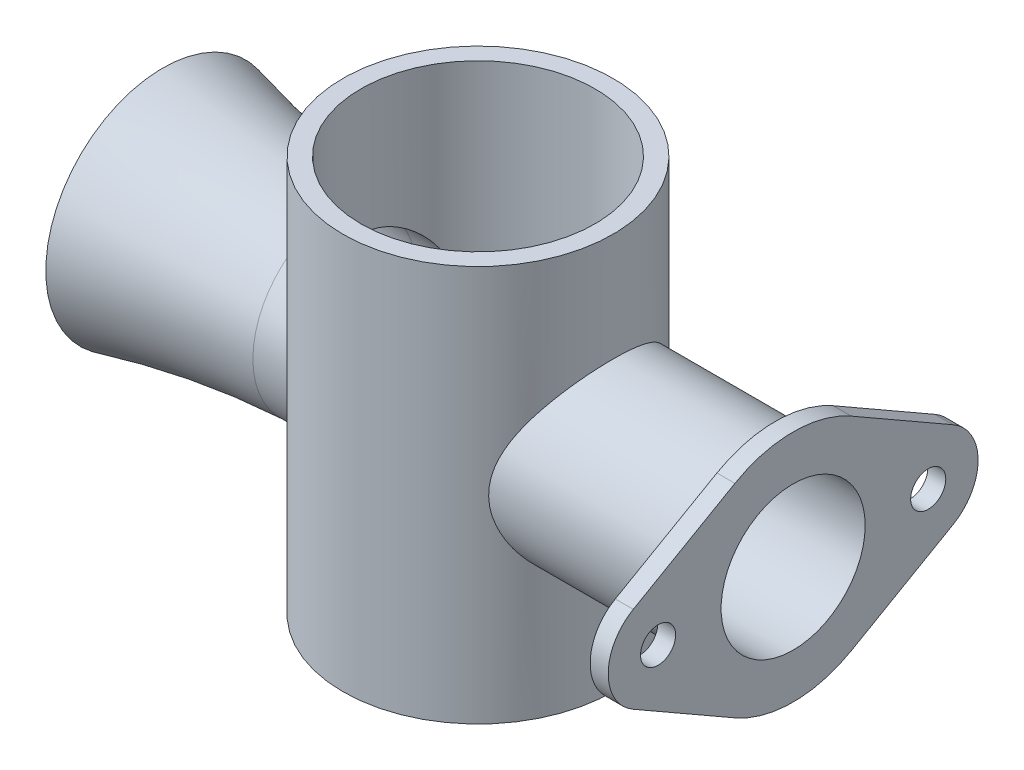
SolidWorks part; units mm, degrees
material "Plain Carbon Steel"
ref_plane "Front Plane" through (0, 0, 0) normal (0, 0, 1) x (1, 0, 0)
ref_plane "Top Plane" through (0, 0, 0) normal (0, 1, 0) x (1, 0, 0)
ref_plane "Right Plane" through (0, 0, 0) normal (1, 0, 0) x (0, 0, -1)
sketch "Main Barrel Sketch" plane through (0, 0, 0) normal (0, 1, 0) x (1, 0, 0)
  circle A0 centre (0, 0) radius 7.5
  circle A1 centre (0, 0) radius 6.5
  dimension "D1" = 15
  dimension "D2" = 13
extrude "Main Barrel" add sketch "Main Barrel Sketch" along normal mid plane 22 contours A0
sketch "Main Bore Sketch Ø13" plane through (0, 11, 0) normal (0, 1, 0) x (1, 0, 0)
  circle A0 centre (0, 0) radius 6.5
  dimension "D1" = 13
extrude "Main Bore Ø13" cut sketch "Main Bore Sketch Ø13" against normal blind 20
ref_plane "Outlet Tube Plane" through (7.5, 0, 0) normal (-1, 0, 0) x (0, 0, 1)
sketch "Outlet Tube Sketch Ø10" plane through (7.5, 0, 0) normal (-1, 0, 0) x (0, 0, 1)
  circle A0 centre (0, 0) radius 5
  dimension "D1" = 10
extrude "Outlet Tube Ø10" add sketch "Outlet Tube Sketch Ø10" against normal blind 9 separate body
sketch "Mounting Flange Sketch" plane through (16.5, 0, 0) normal (1, 0, 0) x (0, 0, -1)
  line L0 (-12.9164, 0) -> (13.3464, 0) construction
  line L1 (-7.5, 11) -> (-7.5, -11) construction
  line L2 (7.5, 11) -> (7.5, -11) construction
  line L3 (0, -9.8134) -> (0, 13.4745) construction
  line L4 (3.2327, 5.6391) -> (8.8776, 2.4031)
  line L5 (3.2327, -5.6391) -> (8.8776, -2.4031)
  line L6 (-3.2327, -5.6391) -> (-8.8776, -2.4031)
  line L7 (-3.2327, 5.6391) -> (-8.8776, 2.4031)
  circle A0 centre (0, 0) radius 4
  arc A1 (3.2327, 5.6391) -> (-3.2327, 5.6391) centre (0, 0) ccw
  circle A2 centre (7.5, 0) radius 0.975
  arc A3 (8.8776, -2.4031) -> (8.8776, 2.4031) centre (7.5, 0) ccw
  arc A4 (-8.8776, -2.4031) -> (-8.8776, 2.4031) centre (-7.5, 0) cw
  arc A5 (-3.2327, -5.6391) -> (3.2327, -5.6391) centre (0, 0) ccw
  circle A6 centre (-7.5, 0) radius 0.975
  dimension "D1" = 8
  dimension "D2" = 13
  dimension "D3" = 1.95
  dimension "D4" = 5.54
extrude "Mounting Flange" add sketch "Mounting Flange Sketch" along normal blind 1
sketch "Outlet Tube Joint Sketch" plane through (7.5, 0, 0) normal (-1, 0, 0) x (0, 0, 1)
  circle A0 centre (0, 0) radius 5 construction
  circle A1 centre (0, 0) radius 5
extrude "Outlet Tube Joint" add sketch "Outlet Tube Joint Sketch" along normal up to surface
ref_plane "Intake Plane" through (-7.5, 0, 0) normal (1, 0, 0) x (0, 0, -1)
sketch "Intake Tube Sketch Ø10" plane through (-7.5, 0, 0) normal (1, 0, 0) x (0, 0, -1)
  circle A0 centre (0, 0) radius 5
  dimension "D1" = 10
sketch "Intake Bell Profile" plane through (0, 0, 0) normal (0, 0, 1) x (1, 0, 0)
  line L0 (-7.5, -5) -> (-7.5, 5) construction
  line L1 (-17.5, 6.5) -> (-17.5, 6)
  line L2 (0, 0) -> (-25.3092, 0) construction
  line L3 (-7.5, 5) -> (-7.5, 4)
  arc A0 (-7.5, 5) -> (-17.5, 6.5) centre (-5.0464, 55.4404) cw
  arc A1 (-17.5, 6) -> (-7.5, 4) centre (-7.5, 30) ccw
  dimension "D3" = 50.5
  dimension "D7" = 26
  dimension "D1" = 5
  dimension "D2" = 6.5
  dimension "D4" = 10
  dimension "D5" = 4
  dimension "D6" = 6
revolve "Intake Bell" add sketch "Intake Bell Profile" angle 360 about L2
extrude "Intake Tube Ø10" add sketch "Intake Tube Sketch Ø10" along normal up to surface up to face at (0, 11, 7.5)
sketch "Outlet Bore Sketch" plane through (16.5, 0, 0) normal (1, 0, 0) x (0, 0, -1)
  circle A0 centre (0, 0) radius 4 construction
  circle A1 centre (0, 0) radius 4
extrude "Outlet Bore" cut sketch "Outlet Bore Sketch" against normal through all
sketch "Side Port Sketch Ø3" plane through (0, -11, 0) normal (0, -1, 0) x (1, 0, 0)
  circle A0 centre (0, 0) radius 1.5
  dimension "D1" = 3
extrude "Side Port Ø3" cut sketch "Side Port Sketch Ø3" against normal blind 2
